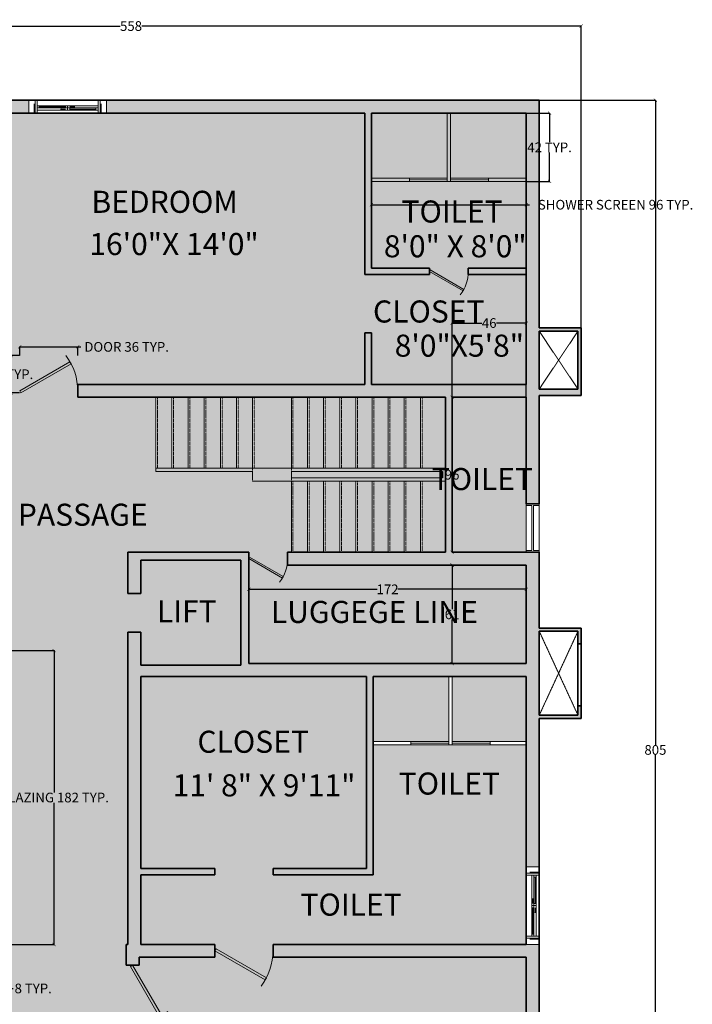
# Model space of a CAD drawing. Units: inches. Extents: x 1704 to 6393, y -157 to 1172.
# Tile 119 of 122: x 4645 to 5062, y 382 to 993. Entities that reach past the tile are written whole.
import ezdxf

# ---------------------------------------------------------------- set-up
doc = ezdxf.new("R2010")
doc.units = ezdxf.units.IN
doc.header["$MEASUREMENT"] = 0
doc.linetypes.add('DASHED', pattern=[0.75, 0.5, -0.25])
doc.linetypes.add('HIDDEN', pattern=[0.375, 0.25, -0.125])
for name, color, linetype, lineweight in [('A-ANNO-DIMS', 7, 'Continuous', 13), ('A-AREA-IDEN', 7, 'Continuous', 18), ('A-FLOR-OPEN-HIDN', 8, 'HIDDEN', 13), ('A-FLOR-STRS-HIDN', 8, 'DASHED', 13), ('A-GLAZ-PATT', 152, 'Continuous', 13), ('A-WALL-PATT', 7, 'Continuous', 13), ('DOORS', 160, 'Continuous', 18), ('GLASS PANEL FASADE', 4, 'Continuous', 18), ('STAIRS', 7, 'Continuous', 18), ('WALLS', 7, 'Continuous', 35), ('WINDOWS', 2, 'Continuous', 18)]:
    doc.layers.add(name, color=color, linetype=linetype, lineweight=lineweight)
doc.layers.add('A-FLOR-PATT', color=7, linetype='Continuous', lineweight=13, true_color=0xf2f2f2)
doc.styles.get("Standard").update_dxf_attribs({"font": 'arial.ttf'})
doc.dimstyles.get("Standard").update_dxf_attribs({"dimtxt": 6, "dimasz": 2, "dimexe": 0.18, "dimexo": 0.0625, "dimgap": 0.09, "dimtad": 0, "dimtih": 1, "dimtoh": 1, "dimdec": 1, "dimzin": 0, "dimdsep": 46, "dimlunit": 3, "dimtxsty": 'Standard', "dimblk": 'ARCHTICK', "dimcen": 0.09, "dimadec": 0, "dimazin": 0, "dimtfac": 1, "dimtdec": 1, "dimtofl": 0, "dimtmove": 0, "dimatfit": 3, "dimfxl": 1, "dimtolj": 1, "dimtzin": 0, "dimarcsym": 0})

# ---------------------------------------------------------------- blocks, each defined once
blk = doc.blocks.new('Door - Left Hung 36 in.')
blk.add_lwpolyline([(0.75, -1.3), (0, 0), (31.18, 18), (31.93, 16.7)], close=True)
blk.add_arc((0, 0), 36, 0, 37.31013)
blk = doc.blocks.new('WIN-SLIDER-48')
for p, q in [((3.83, 8), (0, 8)), ((5.13, 8), (42.87, 8)), ((44.17, 8), (48, 8)), ((3.18, 5.86), (3.18, 0.65)), ((24, 1.95), (5.13, 1.95)), ((6.43, 4.55), (22.7, 4.55)), ((6.43, 3.9), (22.7, 3.9)), ((6.43, 3.25), (22.7, 3.25)), ((22.7, 2.6), (19.9, 2.6)), ((24, 4.55), (42.87, 4.55)), ((25.3, 3.9), (28.1, 3.9)), ((25.3, 3.25), (41.56, 3.25)), ((25.3, 2.6), (41.56, 2.6)), ((25.3, 1.95), (41.56, 1.95)), ((44.82, 5.86), (44.82, 0.65)), ((3.83, 0), (0, 0)), ((5.13, 0), (42.87, 0)), ((44.17, 0), (48, 0))]:
    blk.add_line(p, q)
for points in [[(5.13, 0), (3.83, 0), (3.83, 8), (5.13, 8)], [(42.87, 0), (44.17, 0), (44.17, 8), (42.87, 8)], [(5.13, 3.25), (6.43, 3.25), (6.43, 4.55), (5.13, 4.55)], [(19.57, 2.6), (19.9, 2.8), (19.9, 2.41)], [(22.7, 3.25), (24, 3.25), (24, 4.55), (22.7, 4.55)], [(24, 1.95), (25.3, 1.95), (25.3, 3.25), (24, 3.25)], [(28.43, 3.9), (28.1, 4.1), (28.1, 3.71)], [(41.56, 1.95), (42.87, 1.95), (42.87, 3.25), (41.56, 3.25)]]:
    blk.add_lwpolyline(points, close=True)
blk = doc.blocks.new('WIN-VENT-30')
for p, q in [((0, 0), (0, 30)), ((0, 30), (8, 30)), ((0, 29), (3.5, 29)), ((3.5, 29), (3.5, 1)), ((4.5, 29), (8, 29)), ((4.5, 29), (4.5, 1)), ((8, 30), (8, 0)), ((3.5, 1), (0, 1)), ((8, 1), (4.5, 1)), ((8, 0), (0, 0))]:
    blk.add_line(p, q)
blk = doc.blocks.new('GLAZ-SHOWER-SCREEN-96')
for p, q in [((47, 2), (47, 42.3)), ((49, 2), (49, 42.3)), ((0, 2), (47, 2)), ((23.5, 2), (23.5, 0)), ((23.5, 1), (47, 1)), ((47, 2), (47, 0)), ((49, 2), (96, 2)), ((49, 2), (49, 0)), ((49, 1), (72.5, 1)), ((72.5, 2), (72.5, 0)), ((0, 0), (96, 0))]:
    blk.add_line(p, q)
blk = doc.blocks.new('_ArchTick')
at = {"color": 0, "linetype": 'ByBlock', "const_width": 0.15}
blk.add_lwpolyline([(-0.5, -0.5), (0.5, 0.5)], dxfattribs=at)
blk = doc.blocks.new('*D34')
at = {"layer": 'A-ANNO-DIMS', "color": 0, "lineweight": -2, "transparency": 16777216}
for p, q in [((4645.3, 784.51), (4645.3, 790.02)), ((4645.3, 789.84), (4681.3, 789.84)), ((4681.3, 784.51), (4681.3, 790.02)), ((4681.3, 789.84), (4683.3, 789.84))]:
    blk.add_line(p, q, dxfattribs=at)
at = {"layer": 'Defpoints', "color": 0, "lineweight": -3, "transparency": 16777216}
for p in [(4681.3, 789.84), (4645.3, 784.44), (4681.3, 784.44)]:
    blk.add_point(p, dxfattribs=at)
at = {"layer": 'A-ANNO-DIMS', "color": 0, "lineweight": -2, "transparency": 16777216, "xscale": 2, "yscale": 2, "zscale": 2, "rotation": 180}
blk.add_blockref('_ArchTick', (4645.3, 789.84), dxfattribs=at)
at = {"layer": 'A-ANNO-DIMS', "color": 0, "lineweight": -2, "transparency": 16777216, "xscale": 2, "yscale": 2, "zscale": 2}
blk.add_blockref('_ArchTick', (4681.3, 789.84), dxfattribs=at)
at = {"layer": 'A-ANNO-DIMS', "color": 0, "transparency": 16777216, "insert": (4711.58, 789.84), "char_height": 6, "attachment_point": 5}
blk.add_mtext('\\A1;DOOR 36 TYP.', dxfattribs=at)
blk = doc.blocks.new('*D35')
at = {"layer": 'A-ANNO-DIMS', "color": 0, "lineweight": -2, "transparency": 16777216}
for p, q in [((4645.24, 784.44), (4639.72, 784.44)), ((4639.9, 784.44), (4639.9, 776.04)), ((4639.9, 761.32), (4639.9, 769.73)), ((4645.24, 761.32), (4639.72, 761.32))]:
    blk.add_line(p, q, dxfattribs=at)
at = {"layer": 'Defpoints', "color": 0, "lineweight": -3, "transparency": 16777216}
for p in [(4639.9, 784.44), (4645.3, 784.44), (4645.3, 761.32)]:
    blk.add_point(p, dxfattribs=at)
at = {"layer": 'A-ANNO-DIMS', "color": 0, "lineweight": -2, "transparency": 16777216, "xscale": 2, "yscale": 2, "zscale": 2}
for p, rotation in [((4639.9, 784.44), 90), ((4639.9, 761.32), 270)]:
    blk.add_blockref('_ArchTick', p, dxfattribs=dict(at, rotation=rotation))
at = {"layer": 'A-ANNO-DIMS', "color": 0, "transparency": 16777216, "insert": (4639.9, 772.88), "char_height": 6, "attachment_point": 5}
blk.add_mtext('\\A1;23 TYP.', dxfattribs=at)
blk = doc.blocks.new('*D52')
at = {"layer": 'A-ANNO-DIMS', "color": 0, "lineweight": -2, "transparency": 16777216}
for p, q in [((4639.36, 601.62), (4666.78, 601.62)), ((4666.6, 601.62), (4666.6, 513.82)), ((4666.6, 419.62), (4666.6, 507.43)), ((4639.36, 419.62), (4666.78, 419.62))]:
    blk.add_line(p, q, dxfattribs=at)
at = {"layer": 'Defpoints', "color": 0, "lineweight": -3, "transparency": 16777216}
for p in [(4639.3, 601.62), (4666.6, 601.62), (4639.3, 419.62)]:
    blk.add_point(p, dxfattribs=at)
at = {"layer": 'A-ANNO-DIMS', "color": 0, "lineweight": -2, "transparency": 16777216, "xscale": 2, "yscale": 2, "zscale": 2}
for p, rotation in [((4666.6, 601.62), 90), ((4666.6, 419.62), 270)]:
    blk.add_blockref('_ArchTick', p, dxfattribs=dict(at, rotation=rotation))
at = {"layer": 'A-ANNO-DIMS', "color": 0, "transparency": 16777216, "insert": (4666.6, 510.62), "char_height": 6, "attachment_point": 5}
blk.add_mtext('\\A1;GLAZING 182 TYP.', dxfattribs=at)
blk = doc.blocks.new('*D53')
at = {"layer": 'A-ANNO-DIMS', "color": 0, "lineweight": -2, "transparency": 16777216}
for p, q in [((4631.3, 419.56), (4631.3, 392.14)), ((4639.3, 419.56), (4639.3, 392.14)), ((4631.3, 392.32), (4639.3, 392.32)), ((4639.3, 392.32), (4641.3, 392.32))]:
    blk.add_line(p, q, dxfattribs=at)
at = {"layer": 'Defpoints', "color": 0, "lineweight": -3, "transparency": 16777216}
for p in [(4631.3, 419.62), (4639.3, 419.62), (4639.3, 392.32)]:
    blk.add_point(p, dxfattribs=at)
at = {"layer": 'A-ANNO-DIMS', "color": 0, "lineweight": -2, "transparency": 16777216, "xscale": 2, "yscale": 2, "zscale": 2, "rotation": 180}
blk.add_blockref('_ArchTick', (4631.3, 392.32), dxfattribs=at)
at = {"layer": 'A-ANNO-DIMS', "color": 0, "lineweight": -2, "transparency": 16777216, "xscale": 2, "yscale": 2, "zscale": 2}
blk.add_blockref('_ArchTick', (4639.3, 392.32), dxfattribs=at)
at = {"layer": 'A-ANNO-DIMS', "color": 0, "transparency": 16777216, "insert": (4653.67, 392.32), "char_height": 6, "attachment_point": 5}
blk.add_mtext('\\A1;8 TYP.', dxfattribs=at)
blk = doc.blocks.new('*D54')
at = {"layer": 'A-ANNO-DIMS', "color": 0, "lineweight": -2, "transparency": 16777216}
for p, q in [((4863.3, 892.26), (4863.3, 877.74)), ((4959.3, 892.26), (4959.3, 877.74)), ((4863.3, 877.92), (4959.3, 877.92)), ((4959.3, 877.92), (4961.3, 877.92))]:
    blk.add_line(p, q, dxfattribs=at)
at = {"layer": 'Defpoints', "color": 0, "lineweight": -3, "transparency": 16777216}
for p in [(4863.3, 892.32), (4959.3, 892.32), (4959.3, 877.92)]:
    blk.add_point(p, dxfattribs=at)
at = {"layer": 'A-ANNO-DIMS', "color": 0, "lineweight": -2, "transparency": 16777216, "xscale": 2, "yscale": 2, "zscale": 2, "rotation": 180}
blk.add_blockref('_ArchTick', (4863.3, 877.92), dxfattribs=at)
at = {"layer": 'A-ANNO-DIMS', "color": 0, "lineweight": -2, "transparency": 16777216, "xscale": 2, "yscale": 2, "zscale": 2}
blk.add_blockref('_ArchTick', (4959.3, 877.92), dxfattribs=at)
at = {"layer": 'A-ANNO-DIMS', "color": 0, "transparency": 16777216, "insert": (5014.63, 877.92), "char_height": 6, "attachment_point": 5}
blk.add_mtext('\\A1;SHOWER SCREEN 96 TYP.', dxfattribs=at)
blk = doc.blocks.new('*D55')
at = {"layer": 'A-ANNO-DIMS', "color": 0, "lineweight": -2, "transparency": 16777216}
for p, q in [((4959.36, 934.62), (4973.88, 934.62)), ((4973.7, 934.62), (4973.7, 916.58)), ((4973.7, 892.32), (4973.7, 910.37)), ((4959.36, 892.32), (4973.88, 892.32))]:
    blk.add_line(p, q, dxfattribs=at)
at = {"layer": 'Defpoints', "color": 0, "lineweight": -3, "transparency": 16777216}
for p in [(4959.3, 934.62), (4973.7, 934.62), (4959.3, 892.32)]:
    blk.add_point(p, dxfattribs=at)
at = {"layer": 'A-ANNO-DIMS', "color": 0, "lineweight": -2, "transparency": 16777216, "xscale": 2, "yscale": 2, "zscale": 2}
for p, rotation in [((4973.7, 934.62), 90), ((4973.7, 892.32), 270)]:
    blk.add_blockref('_ArchTick', p, dxfattribs=dict(at, rotation=rotation))
at = {"layer": 'A-ANNO-DIMS', "color": 0, "transparency": 16777216, "insert": (4973.7, 913.47), "char_height": 6, "attachment_point": 5}
blk.add_mtext('\\A1;42 TYP.', dxfattribs=at)
blk = doc.blocks.new('*D107')
at = {"layer": 'A-ANNO-DIMS', "color": 0, "lineweight": -2, "transparency": 16777216}
for p, q in [((4435.3, 942.69), (4435.3, 988.8)), ((4435.3, 988.62), (4707.58, 988.62)), ((4993.3, 988.62), (4721.02, 988.62)), ((4993.3, 801.69), (4993.3, 988.8))]:
    blk.add_line(p, q, dxfattribs=at)
at = {"layer": 'Defpoints', "color": 0, "lineweight": -3, "transparency": 16777216}
for p in [(4993.3, 988.62), (4435.3, 942.62), (4993.3, 801.62)]:
    blk.add_point(p, dxfattribs=at)
at = {"layer": 'A-ANNO-DIMS', "color": 0, "lineweight": -2, "transparency": 16777216, "xscale": 2, "yscale": 2, "zscale": 2, "rotation": 180}
blk.add_blockref('_ArchTick', (4435.3, 988.62), dxfattribs=at)
at = {"layer": 'A-ANNO-DIMS', "color": 0, "lineweight": -2, "transparency": 16777216, "xscale": 2, "yscale": 2, "zscale": 2}
blk.add_blockref('_ArchTick', (4993.3, 988.62), dxfattribs=at)
at = {"layer": 'A-ANNO-DIMS', "color": 0, "transparency": 16777216, "insert": (4714.3, 988.62), "char_height": 6, "attachment_point": 5}
blk.add_mtext('\\A1;558', dxfattribs=at)
blk = doc.blocks.new('*D108')
at = {"layer": 'A-ANNO-DIMS', "color": 0, "lineweight": -2, "transparency": 16777216}
for p, q in [((4967.36, 942.62), (5039.48, 942.62)), ((5039.3, 942.62), (5039.3, 543.28)), ((5039.3, 137.62), (5039.3, 536.97)), ((4967.36, 137.62), (5039.48, 137.62))]:
    blk.add_line(p, q, dxfattribs=at)
at = {"layer": 'Defpoints', "color": 0, "lineweight": -3, "transparency": 16777216}
for p in [(4967.3, 942.62), (5039.3, 942.62), (4967.3, 137.62)]:
    blk.add_point(p, dxfattribs=at)
at = {"layer": 'A-ANNO-DIMS', "color": 0, "lineweight": -2, "transparency": 16777216, "xscale": 2, "yscale": 2, "zscale": 2}
for p, rotation in [((5039.3, 942.62), 90), ((5039.3, 137.62), 270)]:
    blk.add_blockref('_ArchTick', p, dxfattribs=dict(at, rotation=rotation))
at = {"layer": 'A-ANNO-DIMS', "color": 0, "transparency": 16777216, "insert": (5039.3, 540.12), "char_height": 6, "attachment_point": 5}
blk.add_mtext('\\A1;805', dxfattribs=at)
blk = doc.blocks.new('*D115')
at = {"layer": 'A-ANNO-DIMS', "color": 0, "lineweight": -2, "transparency": 16777216}
for p, q in [((4787.3, 593.69), (4787.3, 639.8)), ((4787.3, 639.62), (4866.9, 639.62)), ((4959.3, 639.62), (4879.71, 639.62)), ((4959.3, 593.69), (4959.3, 639.8))]:
    blk.add_line(p, q, dxfattribs=at)
at = {"layer": 'Defpoints', "color": 0, "lineweight": -3, "transparency": 16777216}
for p in [(4959.3, 639.62), (4787.3, 593.62), (4959.3, 593.62)]:
    blk.add_point(p, dxfattribs=at)
at = {"layer": 'A-ANNO-DIMS', "color": 0, "lineweight": -2, "transparency": 16777216, "xscale": 2, "yscale": 2, "zscale": 2, "rotation": 180}
blk.add_blockref('_ArchTick', (4787.3, 639.62), dxfattribs=at)
at = {"layer": 'A-ANNO-DIMS', "color": 0, "lineweight": -2, "transparency": 16777216, "xscale": 2, "yscale": 2, "zscale": 2}
blk.add_blockref('_ArchTick', (4959.3, 639.62), dxfattribs=at)
at = {"layer": 'A-ANNO-DIMS', "color": 0, "transparency": 16777216, "insert": (4873.3, 639.62), "char_height": 6, "attachment_point": 5}
blk.add_mtext('\\A1;172', dxfattribs=at)
blk = doc.blocks.new('*D116')
at = {"layer": 'A-ANNO-DIMS', "color": 0, "lineweight": -2, "transparency": 16777216}
for p, q in [((4959.24, 654.62), (4913.12, 654.62)), ((4913.3, 654.62), (4913.3, 627.28)), ((4913.3, 593.62), (4913.3, 620.97)), ((4959.24, 593.62), (4913.12, 593.62))]:
    blk.add_line(p, q, dxfattribs=at)
at = {"layer": 'Defpoints', "color": 0, "lineweight": -3, "transparency": 16777216}
for p in [(4913.3, 654.62), (4959.3, 654.62), (4959.3, 593.62)]:
    blk.add_point(p, dxfattribs=at)
at = {"layer": 'A-ANNO-DIMS', "color": 0, "lineweight": -2, "transparency": 16777216, "xscale": 2, "yscale": 2, "zscale": 2}
for p, rotation in [((4913.3, 654.62), 90), ((4913.3, 593.62), 270)]:
    blk.add_blockref('_ArchTick', p, dxfattribs=dict(at, rotation=rotation))
at = {"layer": 'A-ANNO-DIMS', "color": 0, "transparency": 16777216, "insert": (4913.3, 624.12), "char_height": 6, "attachment_point": 5}
blk.add_mtext('\\A1;61', dxfattribs=at)
blk = doc.blocks.new('*D117')
at = {"layer": 'A-ANNO-DIMS', "color": 0, "lineweight": -2, "transparency": 16777216}
for p, q in [((4959.24, 758.62), (4913.12, 758.62)), ((4913.3, 758.62), (4913.3, 713.78)), ((4913.3, 662.62), (4913.3, 707.47)), ((4959.24, 662.62), (4913.12, 662.62))]:
    blk.add_line(p, q, dxfattribs=at)
at = {"layer": 'Defpoints', "color": 0, "lineweight": -3, "transparency": 16777216}
for p in [(4913.3, 758.62), (4959.3, 758.62), (4959.3, 662.62)]:
    blk.add_point(p, dxfattribs=at)
at = {"layer": 'A-ANNO-DIMS', "color": 0, "lineweight": -2, "transparency": 16777216, "xscale": 2, "yscale": 2, "zscale": 2}
for p, rotation in [((4913.3, 758.62), 90), ((4913.3, 662.62), 270)]:
    blk.add_blockref('_ArchTick', p, dxfattribs=dict(at, rotation=rotation))
at = {"layer": 'A-ANNO-DIMS', "color": 0, "transparency": 16777216, "insert": (4913.3, 710.62), "char_height": 6, "attachment_point": 5}
blk.add_mtext('\\A1;96', dxfattribs=at)
blk = doc.blocks.new('*D118')
at = {"layer": 'A-ANNO-DIMS', "color": 0, "lineweight": -2, "transparency": 16777216}
for p, q in [((4913.3, 758.69), (4913.3, 804.8)), ((4913.3, 804.62), (4931.79, 804.62)), ((4959.3, 804.62), (4940.81, 804.62)), ((4959.3, 758.69), (4959.3, 804.8))]:
    blk.add_line(p, q, dxfattribs=at)
at = {"layer": 'Defpoints', "color": 0, "lineweight": -3, "transparency": 16777216}
for p in [(4959.3, 804.62), (4913.3, 758.62), (4959.3, 758.62)]:
    blk.add_point(p, dxfattribs=at)
at = {"layer": 'A-ANNO-DIMS', "color": 0, "lineweight": -2, "transparency": 16777216, "xscale": 2, "yscale": 2, "zscale": 2, "rotation": 180}
blk.add_blockref('_ArchTick', (4913.3, 804.62), dxfattribs=at)
at = {"layer": 'A-ANNO-DIMS', "color": 0, "lineweight": -2, "transparency": 16777216, "xscale": 2, "yscale": 2, "zscale": 2}
blk.add_blockref('_ArchTick', (4959.3, 804.62), dxfattribs=at)
at = {"layer": 'A-ANNO-DIMS', "color": 0, "transparency": 16777216, "insert": (4936.3, 804.62), "char_height": 6, "attachment_point": 5}
blk.add_mtext('\\A1;46', dxfattribs=at)
blk = doc.blocks.new('*D138')
at = {"layer": 'A-ANNO-DIMS', "color": 0, "lineweight": -2, "transparency": 16777216}
for p, q in [((4715.21, 406.69), (4715.39, 406.69)), ((4715.3, 406.6), (4715.3, 406.78)), ((4733.73, 352.12), (4726.82, 372.59)), ((4735.73, 352.12), (4733.73, 352.12))]:
    blk.add_line(p, q, dxfattribs=at)
at = {"layer": 'Defpoints', "color": 0, "lineweight": -3, "transparency": 16777216}
for p in [(4715.3, 406.69), (4726.82, 372.59)]:
    blk.add_point(p, dxfattribs=at)
at = {"layer": 'A-ANNO-DIMS', "color": 0, "lineweight": -2, "transparency": 16777216, "xscale": 2, "yscale": 2, "zscale": 2, "rotation": 108.6557587224779}
blk.add_blockref('_ArchTick', (4726.82, 372.59), dxfattribs=at)
at = {"layer": 'A-ANNO-DIMS', "color": 0, "transparency": 16777216, "insert": (4749.48, 352.12), "char_height": 6, "attachment_point": 5}
blk.add_mtext('\\A1;2X R36', dxfattribs=at)

msp = doc.modelspace()

# ---------------------------------------------------------------- hatches: boundary and pattern name
at = {"layer": 'A-FLOR-PATT', "transparency": 33554516}
h = msp.add_hatch(color=256, dxfattribs=at)
h.dxf.hatch_style = 1
h.paths.add_polyline_path([(4859.3, 934.624), (4639.3, 934.624), (4639.3, 766.624), (4645.3, 766.624), (4645.3, 762.624), (4676.477, 780.624), (4677.227, 779.325), (4677.2, 779.309, -0.0929107), (4681.077, 766.624), (4687.3, 766.624), (4859.3, 766.624), (4859.3, 798.624), (4863.3, 798.624), (4863.3, 766.624), (4875.3, 766.624), (4959.3, 766.624), (4959.3, 834.624), (4923.217, 834.624, -0.0999534), (4920.567, 825.5), (4920.585, 825.49), (4920.085, 824.624), (4899.3, 836.624), (4899.3, 834.624), (4863.3, 834.624), (4859.3, 834.624)])
h.paths.add_polyline_path([(4631.3, 890.624), (4443.3, 890.624), (4443.3, 722.624), (4559.3, 722.624), (4559.3, 718.624), (4535.3, 718.624), (4535.3, 712.624), (4531.3, 712.624), (4532.383, 711.999), (4517.396, 686.04, 0.1210664), (4531.3, 682.624), (4535.3, 682.624), (4535.3, 609.624), (4631.3, 609.624), (4631.3, 718.624), (4595.3, 718.624), (4595.3, 722.624), (4631.3, 722.624), (4637.3, 722.624, -0.1140277), (4621.609, 726.711), (4621.593, 726.684), (4620.293, 727.435), (4638.3, 758.624), (4631.3, 758.624)])
h.paths.add_polyline_path([(4531.3, 712.624), (4527.3, 712.624), (4527.3, 718.624), (4443.3, 718.624), (4443.3, 609.624), (4527.3, 609.624), (4527.3, 682.891, -0.0872676), (4517.396, 686.04), (4517.383, 686.018), (4516.3, 686.643)], flags=17)
h.paths.add_polyline_path([(4631.3, 601.624), (4537.3, 510.624), (4631.3, 419.624)], flags=17)
h.paths.add_polyline_path([(4537.3, 510.624), (4443.3, 419.624), (4453.75, 419.624), (4617.46, 419.624), (4631.3, 419.624)], flags=17)
h.paths.add_polyline_path([(4443.3, 601.624), (4443.3, 419.624), (4537.3, 510.624)], flags=17)
h.paths.add_polyline_path([(4631.3, 601.624), (4443.3, 601.624), (4537.3, 510.624)], flags=17)
h.paths.add_polyline_path([(4637.3, 370.694), (4711.3, 370.694), (4715.3, 370.694, 0.1210664), (4731.986, 374.795), (4713.568, 406.694), (4711.3, 406.694), (4711.3, 419.624), (4712.3, 419.624), (4712.3, 613.124), (4720.3, 613.124), (4720.3, 592.624), (4782.3, 592.624), (4782.3, 657.624), (4720.3, 657.624), (4720.3, 637.124), (4712.3, 637.124), (4712.3, 662.624), (4787.3, 662.624), (4787.3, 654.624), (4787.3, 593.624), (4959.3, 593.624), (4959.3, 654.624), (4811.3, 654.624), (4811.3, 662.624), (4813.69, 662.624), (4813.69, 706.624), (4789.69, 706.624), (4789.69, 712.624), (4729.69, 712.624), (4729.69, 714.624), (4729.69, 758.624), (4681.3, 758.624), (4681.3, 762.624, 0.1210664), (4677.2, 779.309), (4645.3, 760.892), (4645.3, 758.624), (4638.3, 758.624), (4639.6, 757.873), (4621.609, 726.711, 0.1140277), (4637.3, 722.624), (4639.3, 722.624), (4639.3, 601.624), (4639.3, 419.624), (4639.3, 411.624), (4617.46, 411.624), (4453.75, 411.624), (4443.3, 411.624), (4443.3, 249.624), (4637.3, 249.624)])
h.paths.add_polyline_path([(4813.69, 758.624), (4790.69, 758.624), (4790.69, 714.624), (4813.69, 714.624)], flags=17)
h.paths.add_polyline_path([(4789.69, 758.624), (4780.69, 758.624), (4780.69, 714.624), (4789.69, 714.624)], flags=17)
h.paths.add_polyline_path([(4779.69, 758.624), (4770.69, 758.624), (4770.69, 714.624), (4779.69, 714.624)], flags=17)
h.paths.add_polyline_path([(4769.69, 758.624), (4760.69, 758.624), (4760.69, 714.624), (4769.69, 714.624)], flags=17)
h.paths.add_polyline_path([(4759.69, 758.624), (4750.69, 758.624), (4750.69, 714.624), (4759.69, 714.624)], flags=17)
h.paths.add_polyline_path([(4749.69, 758.624), (4740.69, 758.624), (4740.69, 714.624), (4749.69, 714.624)], flags=17)
h.paths.add_polyline_path([(4739.69, 758.624), (4730.69, 758.624), (4730.69, 714.624), (4739.69, 714.624)], flags=17)
h.paths.add_polyline_path([(4823.69, 758.624), (4814.69, 758.624), (4814.69, 714.624), (4823.69, 714.624)], flags=17)
h.paths.add_polyline_path([(4833.69, 758.624), (4824.69, 758.624), (4824.69, 714.624), (4833.69, 714.624)], flags=17)
h.paths.add_polyline_path([(4843.69, 758.624), (4834.69, 758.624), (4834.69, 714.624), (4843.69, 714.624)], flags=17)
h.paths.add_polyline_path([(4909.3, 706.624), (4894.69, 706.624), (4894.69, 662.624), (4909.3, 662.624)], flags=17)
h.paths.add_polyline_path([(4883.69, 706.624), (4874.69, 706.624), (4874.69, 662.624), (4883.69, 662.624)], flags=17)
h.paths.add_polyline_path([(4853.69, 706.624), (4844.69, 706.624), (4844.69, 662.624), (4853.69, 662.624)], flags=17)
h.paths.add_polyline_path([(4833.69, 706.624), (4824.69, 706.624), (4824.69, 662.624), (4833.69, 662.624)], flags=17)
h.paths.add_polyline_path([(4823.69, 706.624), (4814.69, 706.624), (4814.69, 662.624), (4823.69, 662.624)], flags=17)
h.paths.add_polyline_path([(4843.69, 706.624), (4834.69, 706.624), (4834.69, 662.624), (4843.69, 662.624)], flags=17)
h.paths.add_polyline_path([(4863.69, 706.624), (4854.69, 706.624), (4854.69, 662.624), (4863.69, 662.624)], flags=17)
h.paths.add_polyline_path([(4873.69, 706.624), (4864.69, 706.624), (4864.69, 662.624), (4873.69, 662.624)], flags=17)
h.paths.add_polyline_path([(4893.69, 706.624), (4884.69, 706.624), (4884.69, 662.624), (4893.69, 662.624)], flags=17)
h.paths.add_polyline_path([(4853.69, 758.624), (4844.69, 758.624), (4844.69, 714.624), (4853.69, 714.624)], flags=17)
h.paths.add_polyline_path([(4873.69, 758.624), (4864.69, 758.624), (4864.69, 714.624), (4873.69, 714.624)], flags=17)
h.paths.add_polyline_path([(4893.69, 758.624), (4884.69, 758.624), (4884.69, 714.624), (4893.69, 714.624)], flags=17)
h.paths.add_polyline_path([(4909.3, 758.624), (4894.69, 758.624), (4894.69, 714.624), (4909.3, 714.624)], flags=17)
h.paths.add_polyline_path([(4863.69, 758.624), (4854.69, 758.624), (4854.69, 714.624), (4863.69, 714.624)], flags=17)
h.paths.add_polyline_path([(4883.69, 758.624), (4874.69, 758.624), (4874.69, 714.624), (4883.69, 714.624)], flags=17)
h.paths.add_polyline_path([(4907.3, 712.624), (4813.69, 712.624), (4813.69, 708.624), (4907.3, 708.624)], flags=17)
at = {"layer": 'A-FLOR-PATT', "transparency": 33554511}
h = msp.add_hatch(color=256, dxfattribs=at)
h.dxf.hatch_style = 1
h.paths.add_polyline_path([(4860.3, 585.624), (4839.3, 585.624), (4720.3, 585.624), (4720.3, 466.624), (4766.3, 466.624), (4766.3, 462.624), (4720.3, 462.624), (4720.3, 419.624), (4766.3, 419.624), (4766.3, 415.624), (4767.05, 416.923), (4798.2, 398.938, 0.1210664), (4802.3, 415.624), (4802.3, 419.624), (4959.3, 419.624), (4959.3, 423.456), (4959.3, 424.757), (4959.3, 462.49), (4959.3, 463.791), (4959.3, 467.624), (4959.3, 543.32), (4864.3, 543.32), (4864.3, 462.624), (4802.3, 462.624), (4802.3, 466.624), (4860.3, 466.624)], flags=17)
h.paths.add_polyline_path([(4959.3, 411.624), (4802.077, 411.624, -0.0929107), (4798.2, 398.938), (4767.05, 416.923), (4766.3, 415.624), (4766.3, 411.624), (4719.3, 411.624), (4719.3, 406.694), (4711.3, 406.694), (4711.3, 419.624), (4712.3, 419.624), (4712.3, 613.124), (4720.3, 613.124), (4720.3, 592.624), (4782.3, 592.624), (4782.3, 657.624), (4720.3, 657.624), (4720.3, 637.124), (4712.3, 637.124), (4712.3, 662.624), (4787.3, 662.624), (4787.3, 654.624), (4787.3, 593.624), (4959.3, 593.624), (4959.3, 654.624), (4811.3, 654.624), (4811.3, 662.624), (4813.69, 662.624), (4813.69, 706.624), (4789.69, 706.624), (4789.69, 712.624), (4729.69, 712.624), (4729.69, 714.624), (4729.69, 758.624), (4681.3, 758.624), (4681.3, 766.624), (4687.3, 766.624), (4859.3, 766.624), (4859.3, 798.624), (4863.3, 798.624), (4863.3, 766.624), (4875.3, 766.624), (4959.3, 766.624), (4959.3, 834.624), (4923.3, 834.624), (4923.3, 838.624), (4959.3, 838.624), (4959.3, 892.32), (4863.3, 892.32), (4863.3, 838.624), (4899.3, 838.624), (4899.3, 834.624), (4863.3, 834.624), (4859.3, 834.624), (4859.3, 934.624), (4639.3, 934.624), (4639.3, 766.624), (4645.3, 766.624), (4645.3, 758.624), (4631.3, 758.624), (4631.3, 890.624), (4443.3, 890.624), (4443.3, 722.624), (4559.3, 722.624), (4559.3, 718.624), (4535.3, 718.624), (4535.3, 712.624), (4527.3, 712.624), (4527.3, 718.624), (4443.3, 718.624), (4443.3, 609.624), (4527.3, 609.624), (4527.3, 682.624), (4535.3, 682.624), (4535.3, 609.624), (4631.3, 609.624), (4631.3, 718.624), (4595.3, 718.624), (4595.3, 722.624), (4631.3, 722.624), (4639.3, 722.624), (4639.3, 601.624), (4639.3, 419.624), (4639.3, 411.624), (4617.46, 411.624), (4453.75, 411.624), (4443.3, 411.624), (4443.3, 249.624), (4637.3, 249.624), (4637.3, 370.694), (4711.3, 370.694), (4719.3, 370.694), (4719.3, 145.624), (4959.3, 145.624), (4959.3, 265.624)])
h.paths.add_polyline_path([(4645.3, 362.694), (4645.3, 249.624), (4678.295, 306.15)], flags=17)
h.paths.add_polyline_path([(4711.3, 362.694), (4645.3, 362.694), (4678.295, 306.15)], flags=17)
h.paths.add_polyline_path([(4711.3, 362.694), (4678.295, 306.15), (4711.279, 249.624), (4711.3, 249.624)], flags=17)
at = {"layer": 'A-FLOR-PATT', "transparency": 33554559}
h = msp.add_hatch(color=256, dxfattribs=at)
h.dxf.hatch_style = 1
h.paths.add_polyline_path([(4959.3, 892.32), (4863.3, 892.32), (4863.3, 838.624), (4899.3, 838.624), (4899.3, 836.624), (4899.8, 837.49), (4920.567, 825.5, 0.1210664), (4923.3, 836.624), (4923.3, 838.624), (4959.3, 838.624)])
h.paths.add_polyline_path([(4910.3, 934.624), (4863.3, 934.624), (4863.3, 894.32), (4910.3, 894.32)])
h.paths.add_polyline_path([(4959.3, 934.624), (4912.3, 934.624), (4912.3, 894.32), (4959.3, 894.32)])
h = msp.add_hatch(color=256, dxfattribs=at)
h.dxf.hatch_style = 1
h.paths.add_polyline_path([(4959.3, 758.624), (4913.3, 758.624), (4913.3, 662.624), (4959.3, 662.624), (4959.3, 692.624)])
h = msp.add_hatch(color=256, dxfattribs=at)
h.dxf.hatch_style = 1
h.paths.add_polyline_path([(4911.3, 585.624), (4864.3, 585.624), (4864.3, 545.32), (4911.3, 545.32)])
h.paths.add_polyline_path([(4959.3, 585.624), (4913.3, 585.624), (4913.3, 545.32), (4959.3, 545.32)])
at = {"layer": 'A-GLAZ-PATT', "transparency": 33554559}
h = msp.add_hatch(color=256, dxfattribs=at)
h.dxf.hatch_style = 1
h.paths.add_polyline_path([(4886.8, 894.32), (4863.3, 894.32), (4863.3, 892.32), (4886.8, 892.32)])
h.paths.add_polyline_path([(4912.3, 934.624), (4910.3, 934.624), (4910.3, 894.32), (4910.3, 892.32), (4912.3, 892.32), (4912.3, 894.32)])
h = msp.add_hatch(color=256, dxfattribs=at)
h.dxf.hatch_style = 1
h.paths.add_polyline_path([(4959.3, 894.32), (4935.8, 894.32), (4935.8, 892.32), (4959.3, 892.32)])
at = {"layer": 'A-WALL-PATT'}
h = msp.add_hatch(color=256, dxfattribs=at)
h.dxf.hatch_style = 1
h.paths.add_polyline_path([(4967.3, 942.624), (4699.009, 942.624), (4699.009, 934.624), (4859.3, 934.624), (4859.3, 834.624), (4863.3, 834.624), (4899.3, 834.624), (4899.3, 838.624), (4863.3, 838.624), (4863.3, 934.624), (4959.3, 934.624), (4959.3, 901.624), (4959.3, 834.624), (4959.3, 766.624), (4863.3, 766.624), (4863.3, 798.624), (4859.3, 798.624), (4859.3, 766.624), (4687.3, 766.624), (4681.3, 766.624), (4681.3, 758.624), (4909.3, 758.624), (4909.3, 662.624), (4811.3, 662.624), (4811.3, 654.624), (4959.3, 654.624), (4959.3, 593.624), (4787.3, 593.624), (4787.3, 654.624), (4787.3, 662.624), (4712.3, 662.624), (4712.3, 637.124), (4720.3, 637.124), (4720.3, 657.624), (4782.3, 657.624), (4782.3, 592.624), (4720.3, 592.624), (4720.3, 613.124), (4712.3, 613.124), (4712.3, 419.624), (4711.3, 419.624), (4711.3, 406.694), (4719.3, 406.694), (4719.3, 411.624), (4766.3, 411.624), (4766.3, 419.624), (4720.3, 419.624), (4720.3, 462.624), (4766.3, 462.624), (4766.3, 466.624), (4720.3, 466.624), (4720.3, 585.624), (4839.3, 585.624), (4860.3, 585.624), (4860.3, 466.624), (4802.3, 466.624), (4802.3, 462.624), (4864.3, 462.624), (4864.3, 585.624), (4959.3, 585.624), (4959.3, 542.624), (4959.3, 467.624), (4967.3, 467.624), (4967.3, 559.624), (4993.3, 559.624), (4993.3, 567.435), (4991.3, 567.435), (4991.3, 561.624), (4967.3, 561.624), (4967.3, 613.624), (4991.3, 613.624), (4991.3, 605.789), (4993.3, 605.789), (4993.3, 615.624), (4967.3, 615.624), (4967.3, 654.624), (4967.3, 662.624), (4959.3, 662.624), (4913.3, 662.624), (4913.3, 758.624), (4959.3, 758.624), (4959.3, 692.624), (4967.3, 692.624), (4967.3, 759.624), (4993.3, 759.624), (4993.3, 801.624), (4967.3, 801.624)])
h.paths.add_polyline_path([(4967.3, 799.624), (4991.3, 799.624), (4991.3, 763.624), (4967.3, 763.624)], flags=16)
h.paths.add_polyline_path([(4443.3, 718.624), (4527.3, 718.624), (4527.3, 712.624), (4535.3, 712.624), (4535.3, 718.624), (4559.3, 718.624), (4559.3, 722.624), (4443.3, 722.624), (4435.3, 722.624), (4435.3, 601.624), (4443.3, 601.624), (4639.3, 601.624), (4639.3, 722.624), (4631.3, 722.624), (4595.3, 722.624), (4595.3, 718.624), (4631.3, 718.624), (4631.3, 609.624), (4535.3, 609.624), (4535.3, 682.624), (4527.3, 682.624), (4527.3, 609.624), (4443.3, 609.624)])
h.paths.add_polyline_path([(4443.3, 890.624), (4489.3, 890.624), (4489.3, 898.624), (4443.3, 898.624), (4443.3, 934.624), (4455.446, 934.624), (4455.446, 942.624), (4435.3, 942.624), (4435.3, 794.624), (4443.3, 794.624)])
h.paths.add_polyline_path([(4639.3, 934.624), (4651.009, 934.624), (4651.009, 942.624), (4635.3, 942.624), (4619.155, 942.624), (4619.155, 934.624), (4631.3, 934.624), (4631.3, 898.624), (4585.3, 898.624), (4585.3, 890.624), (4631.3, 890.624), (4631.3, 758.624), (4645.3, 758.624), (4645.3, 766.624), (4639.3, 766.624)])
h.paths.add_polyline_path([(4967.3, 265.624), (4967.3, 309.624), (4959.3, 309.624), (4959.3, 265.624), (4959.3, 145.624), (4719.3, 145.624), (4719.3, 370.694), (4711.3, 370.694), (4711.3, 249.624), (4699.3, 249.624), (4651.3, 249.624), (4639.3, 249.624), (4585.307, 249.624), (4585.307, 241.624), (4639.3, 241.624), (4651.3, 241.624), (4699.3, 241.624), (4711.3, 241.624), (4711.3, 137.624), (4719.3, 137.624), (4959.3, 137.624), (4967.3, 137.624)])
h.paths.add_polyline_path([(4489.307, 249.624), (4435.313, 249.624), (4435.313, 241.624), (4489.307, 241.624)])
h.paths.add_polyline_path([(4967.3, 419.624), (4959.3, 419.624), (4802.3, 419.624), (4802.3, 411.624), (4959.3, 411.624), (4959.3, 381.624), (4967.3, 381.624)])
h.paths.add_polyline_path([(4967.3, 381.624), (4959.3, 381.624), (4959.3, 376.851), (4967.3, 376.851)])
h.paths.add_polyline_path([(4967.3, 314.396), (4959.3, 314.396), (4959.3, 309.624), (4967.3, 309.624)], flags=17)
h.paths.add_polyline_path([(4959.3, 838.624), (4923.3, 838.624), (4923.3, 834.624), (4959.3, 834.624)], flags=17)
h = msp.add_hatch(color=256, dxfattribs=at)
h.dxf.hatch_style = 1
h.paths.add_polyline_path([(4813.69, 714.624), (4789.69, 714.624), (4789.69, 706.624), (4813.69, 706.624)])
h.paths.add_polyline_path([(4909.3, 714.624), (4813.69, 714.624), (4813.69, 712.624), (4907.3, 712.624), (4907.3, 708.624), (4813.69, 708.624), (4813.69, 706.624), (4909.3, 706.624)])
h.paths.add_polyline_path([(4789.69, 714.624), (4729.69, 714.624), (4729.69, 712.624), (4789.69, 712.624)])

# ---------------------------------------------------------------- linework, layer by layer
at = {"layer": 'A-FLOR-OPEN-HIDN'}
for p, q in [((4967.3, 763.624), (4991.3, 799.624)), ((4967.3, 799.624), (4991.3, 763.624)), ((4967.3, 561.624), (4991.3, 613.624)), ((4967.3, 613.624), (4991.3, 561.624))]:
    msp.add_line(p, q, dxfattribs=at)
at = {"layer": 'A-FLOR-STRS-HIDN'}
for p, q in [((4730.69, 714.624), (4730.69, 758.624)), ((4740.69, 714.624), (4740.69, 758.624)), ((4750.69, 714.624), (4750.69, 758.624)), ((4760.69, 714.624), (4760.69, 758.624)), ((4770.69, 714.624), (4770.69, 758.624)), ((4780.69, 714.624), (4780.69, 758.624)), ((4790.69, 714.624), (4790.69, 758.624)), ((4814.69, 714.624), (4814.69, 758.624)), ((4824.69, 714.624), (4824.69, 758.624)), ((4834.69, 714.624), (4834.69, 758.624)), ((4844.69, 714.624), (4844.69, 758.624)), ((4854.69, 714.624), (4854.69, 758.624)), ((4864.69, 714.624), (4864.69, 758.624)), ((4874.69, 714.624), (4874.69, 758.624)), ((4884.69, 714.624), (4884.69, 758.624)), ((4894.69, 714.624), (4894.69, 758.624)), ((4789.69, 714.624), (4789.69, 706.624)), ((4813.69, 706.624), (4813.69, 714.624)), ((4814.69, 706.624), (4814.69, 662.624)), ((4824.69, 706.624), (4824.69, 662.624)), ((4834.69, 706.624), (4834.69, 662.624)), ((4844.69, 706.624), (4844.69, 662.624)), ((4854.69, 706.624), (4854.69, 662.624)), ((4864.69, 706.624), (4864.69, 662.624)), ((4874.69, 706.624), (4874.69, 662.624)), ((4884.69, 706.624), (4884.69, 662.624)), ((4894.69, 706.624), (4894.69, 662.624))]:
    msp.add_line(p, q, dxfattribs=at)
at = {"layer": 'GLASS PANEL FASADE'}
for p, q in [((4911.3, 545.32), (4911.3, 585.624)), ((4913.3, 545.32), (4913.3, 585.624)), ((4864.3, 545.32), (4911.3, 545.32)), ((4864.3, 543.32), (4959.3, 543.32)), ((4887.8, 543.32), (4887.8, 545.32)), ((4887.8, 544.32), (4911.3, 544.32)), ((4911.3, 545.32), (4911.3, 543.32)), ((4913.3, 545.32), (4959.3, 545.32)), ((4913.3, 545.32), (4913.3, 543.32)), ((4913.3, 544.32), (4936.8, 544.32)), ((4936.8, 543.32), (4936.8, 545.32))]:
    msp.add_line(p, q, dxfattribs=at)
at = {"layer": 'STAIRS'}
for p, q in [((4729.69, 714.624), (4729.69, 758.624)), ((4739.69, 714.624), (4739.69, 758.624)), ((4749.69, 714.624), (4749.69, 758.624)), ((4759.69, 714.624), (4759.69, 758.624)), ((4769.69, 714.624), (4769.69, 758.624)), ((4779.69, 714.624), (4779.69, 758.624)), ((4789.69, 714.624), (4789.69, 758.624)), ((4813.69, 714.624), (4813.69, 758.624)), ((4823.69, 714.624), (4823.69, 758.624)), ((4833.69, 714.624), (4833.69, 758.624)), ((4843.69, 714.624), (4843.69, 758.624)), ((4853.69, 714.624), (4853.69, 758.624)), ((4863.69, 714.624), (4863.69, 758.624)), ((4873.69, 714.624), (4873.69, 758.624)), ((4883.69, 714.624), (4883.69, 758.624)), ((4893.69, 714.624), (4893.69, 758.624)), ((4909.3, 714.624), (4729.69, 714.624)), ((4729.69, 712.624), (4729.69, 714.624)), ((4789.69, 712.624), (4729.69, 712.624)), ((4907.3, 712.624), (4813.69, 712.624)), ((4907.3, 708.624), (4813.69, 708.624)), ((4909.3, 706.624), (4789.69, 706.624)), ((4813.69, 706.624), (4813.69, 662.624)), ((4823.69, 706.624), (4823.69, 662.624)), ((4833.69, 706.624), (4833.69, 662.624)), ((4843.69, 706.624), (4843.69, 662.624)), ((4853.69, 706.624), (4853.69, 662.624)), ((4863.69, 706.624), (4863.69, 662.624)), ((4873.69, 706.624), (4873.69, 662.624)), ((4883.69, 706.624), (4883.69, 662.624)), ((4893.69, 706.624), (4893.69, 662.624))]:
    msp.add_line(p, q, dxfattribs=at)
at = {"layer": 'WALLS'}
for p, q in [((4967.3, 942.624), (4435.3, 942.624)), ((4967.3, 942.624), (4635.3, 942.624)), ((4967.3, 942.624), (4943.3, 942.624)), ((4967.3, 801.624), (4967.3, 942.624)), ((4967.3, 901.624), (4967.3, 942.624)), ((4859.3, 934.624), (4639.3, 934.624)), ((4859.3, 934.624), (4695.3, 934.624)), ((4859.3, 834.624), (4859.3, 934.624)), ((4959.3, 934.624), (4863.3, 934.624)), ((4863.3, 838.624), (4863.3, 934.624)), ((4863.3, 838.624), (4863.3, 934.624)), ((4959.3, 934.624), (4943.3, 934.624)), ((4959.3, 834.624), (4959.3, 934.624)), ((4959.3, 901.624), (4959.3, 934.624)), ((4959.3, 766.624), (4959.3, 865.624)), ((4899.3, 838.624), (4863.3, 838.624)), ((4899.3, 834.624), (4899.3, 838.624)), ((4959.3, 838.624), (4923.3, 838.624)), ((4923.3, 834.624), (4923.3, 838.624)), ((4863.3, 834.624), (4859.3, 834.624)), ((4899.3, 834.624), (4863.3, 834.624)), ((4959.3, 834.624), (4923.3, 834.624)), ((4967.3, 801.624), (4993.3, 801.624)), ((4967.3, 763.624), (4967.3, 799.624)), ((4967.3, 799.624), (4991.3, 799.624)), ((4991.3, 799.624), (4991.3, 763.624)), ((4993.3, 801.624), (4993.3, 759.624)), ((4859.3, 766.624), (4859.3, 798.624)), ((4863.3, 798.624), (4859.3, 798.624)), ((4863.3, 766.624), (4863.3, 798.624)), ((4687.3, 766.624), (4681.3, 766.624)), ((4681.3, 766.624), (4681.3, 758.624)), ((4859.3, 766.624), (4687.3, 766.624)), ((4959.3, 766.624), (4863.3, 766.624)), ((4875.3, 766.624), (4863.3, 766.624)), ((4967.3, 763.624), (4991.3, 763.624)), ((4909.3, 758.624), (4681.3, 758.624)), ((4909.3, 662.624), (4909.3, 758.624)), ((4913.3, 662.624), (4913.3, 758.624)), ((4959.3, 758.624), (4913.3, 758.624)), ((4959.3, 692.624), (4959.3, 758.624)), ((4967.3, 692.624), (4967.3, 759.624)), ((4967.3, 759.624), (4993.3, 759.624)), ((4907.3, 708.624), (4907.3, 712.624)), ((4959.3, 692.624), (4967.3, 692.624)), ((4712.3, 637.124), (4712.3, 662.624)), ((4787.3, 662.624), (4712.3, 662.624)), ((4787.3, 654.624), (4787.3, 662.624)), ((4909.3, 662.624), (4811.3, 662.624)), ((4811.3, 654.624), (4811.3, 662.624)), ((4959.3, 662.624), (4913.3, 662.624)), ((4959.3, 662.624), (4967.3, 662.624)), ((4967.3, 654.624), (4967.3, 662.624)), ((4720.3, 637.124), (4720.3, 657.624)), ((4782.3, 657.624), (4720.3, 657.624)), ((4782.3, 592.624), (4782.3, 657.624)), ((4787.3, 593.624), (4787.3, 654.624)), ((4959.3, 654.624), (4811.3, 654.624)), ((4894.3, 654.624), (4880.3, 654.624)), ((4959.3, 654.624), (4894.3, 654.624)), ((4959.3, 593.624), (4959.3, 654.624)), ((4967.3, 615.624), (4967.3, 654.624)), ((4720.3, 637.124), (4712.3, 637.124)), ((4712.3, 419.624), (4712.3, 613.124)), ((4720.3, 613.124), (4712.3, 613.124)), ((4720.3, 592.624), (4720.3, 613.124)), ((4967.3, 615.624), (4993.3, 615.624)), ((4967.3, 561.624), (4967.3, 613.624)), ((4967.3, 613.624), (4991.3, 613.624)), ((4991.3, 613.624), (4991.3, 561.624)), ((4993.3, 615.624), (4993.3, 559.624)), ((4991.3, 605.789), (4993.3, 605.789)), ((4782.3, 592.624), (4720.3, 592.624)), ((4959.3, 593.624), (4787.3, 593.624)), ((4876.3, 593.624), (4864.3, 593.624)), ((4839.3, 585.624), (4720.3, 585.624)), ((4720.3, 466.624), (4720.3, 585.624)), ((4860.3, 585.624), (4839.3, 585.624)), ((4860.3, 466.624), (4860.3, 585.624)), ((4959.3, 585.624), (4864.3, 585.624)), ((4864.3, 462.624), (4864.3, 585.624)), ((4959.3, 542.624), (4959.3, 585.624)), ((4959.3, 419.624), (4959.3, 585.624)), ((4991.3, 567.435), (4993.3, 567.435)), ((4967.3, 561.624), (4991.3, 561.624)), ((4967.3, 265.624), (4967.3, 559.624)), ((4967.3, 542.624), (4967.3, 559.624)), ((4967.3, 559.624), (4993.3, 559.624)), ((4766.3, 466.624), (4720.3, 466.624)), ((4766.3, 466.624), (4766.3, 462.624)), ((4860.3, 466.624), (4802.3, 466.624)), ((4802.3, 466.624), (4802.3, 462.624)), ((4720.3, 419.624), (4720.3, 462.624)), ((4766.3, 462.624), (4720.3, 462.624)), ((4864.3, 462.624), (4802.3, 462.624)), ((4711.3, 406.694), (4711.3, 419.624)), ((4712.3, 419.624), (4711.3, 419.624)), ((4766.3, 419.624), (4720.3, 419.624)), ((4766.3, 419.624), (4766.3, 411.624)), ((4959.3, 419.624), (4802.3, 419.624)), ((4802.3, 419.624), (4802.3, 411.624)), ((4719.3, 406.694), (4719.3, 411.624)), ((4766.3, 411.624), (4719.3, 411.624)), ((4959.3, 411.624), (4802.3, 411.624)), ((4959.3, 265.624), (4959.3, 411.624)), ((4959.3, 375.624), (4959.3, 411.624)), ((4711.3, 406.694), (4719.3, 406.694))]:
    msp.add_line(p, q, dxfattribs=at)
at = {"layer": 'WINDOWS'}
for p, q in [((4651.009, 942.624), (4651.009, 934.624)), ((4699.009, 942.624), (4699.009, 934.624)), ((4967.3, 467.624), (4959.3, 467.624)), ((4967.3, 419.624), (4959.3, 419.624))]:
    msp.add_line(p, q, dxfattribs=at)

# ---------------------------------------------------------------- block references
at = {"layer": 'DOORS', "xscale": -0.666666666666667, "yscale": 0.666666666666667, "zscale": 0.666666666666667, "rotation": 180}
for p in [(4899.3, 836.624), (4787.3, 658.624)]:
    msp.add_blockref('Door - Left Hung 36 in.', p, dxfattribs=at)
at = {"layer": 'DOORS'}
msp.add_blockref('Door - Left Hung 36 in.', (4645.3, 762.624), dxfattribs=at)
at = {"layer": 'DOORS', "xscale": -1, "rotation": 180}
msp.add_blockref('Door - Left Hung 36 in.', (4766.3, 415.624), dxfattribs=at)
at = {"layer": 'DOORS', "rotation": 270}
msp.add_blockref('Door - Left Hung 36 in.', (4715.3, 406.694), dxfattribs=at)
at = {"layer": 'GLASS PANEL FASADE'}
msp.add_blockref('GLAZ-SHOWER-SCREEN-96', (4863.3, 892.32), dxfattribs=at)
at = {"layer": 'WINDOWS'}
for name, p in [('WIN-SLIDER-48', (4651.01, 934.624)), ('WIN-VENT-30', (4959.3, 662.624))]:
    msp.add_blockref(name, p, dxfattribs=at)
at = {"layer": 'WINDOWS', "rotation": 90.00000000000254}
msp.add_blockref('WIN-SLIDER-48', (4967.3, 419.624), dxfattribs=at)

# ---------------------------------------------------------------- texts
at = {"layer": 'A-ANNO-DIMS'}
for s, p in [('16\'0"X 14\'0"', (4688.442, 846.715)), ('8\'0" X 8\'0"', (4871.014, 845.334)), ('8\'0"X5\'8"', (4877.718, 783.758)), ('11\' 8" X 9\'11"', (4740.041, 511.331))]:
    msp.add_text(s, height=13.6672, dxfattribs=at).set_placement(p)
at = {"layer": 'A-AREA-IDEN'}
for s, p in [('BEDROOM', (4689.781, 872.885)), ('TOILET', (4881.929, 866.87)), ('CLOSET', (4864.257, 804.924)), ('TOILET', (4900.683, 701.098)), ('PASSAGE', (4644.149, 679.012)), ('LIFT', (4730.33, 619.179)), ('LUGGEGE LINE', (4800.939, 618.79)), ('CLOSET', (4755.444, 538.343)), ('TOILET', (4880.202, 512.442)), ('TOILET', (4819.351, 437.436))]:
    msp.add_text(s, height=13.6672, dxfattribs=at).set_placement(p)

# ---------------------------------------------------------------- dimensions: what is measured, and where the dimension line sits
at = {"layer": 'A-ANNO-DIMS'}
for base, p1, p2, picture, middle in [((4993.3, 988.624), (4435.3, 942.624), (4993.3, 801.624), '*D107', (4714.3, 988.624)), ((4959.3, 639.624), (4787.3, 593.624), (4959.3, 593.624), '*D115', (4873.3, 639.624))]:
    dim = msp.add_linear_dim(base=base, p1=p1, p2=p2, dimstyle='Standard', override={"dimdec": 0, "dimlfac": 1, "dimrnd": 0, "dimzin": 0, "dimdsep": 46, "dimlunit": 2}, dxfattribs=at)
    dim.commit()
    dim.dimension.update_dxf_attribs({"geometry": picture, "text_midpoint": middle})
for base, p1, p2, angle, picture, middle in [((5039.3, 942.624), (4967.3, 137.624), (4967.3, 942.624), 90, '*D108', (5039.3, 540.124)), ((4959.3, 804.624), (4913.3, 758.624), (4959.3, 758.624), 0, '*D118', (4936.3, 804.624)), ((4913.3, 758.624), (4959.3, 662.624), (4959.3, 758.624), 90, '*D117', (4913.3, 710.624)), ((4913.3, 654.624), (4959.3, 593.624), (4959.3, 654.624), 90, '*D116', (4913.3, 624.124))]:
    dim = msp.add_linear_dim(base=base, p1=p1, p2=p2, angle=angle, dimstyle='Standard', override={"dimdec": 0, "dimlfac": 1, "dimrnd": 0, "dimzin": 0, "dimdsep": 46, "dimlunit": 2}, dxfattribs=at)
    dim.commit()
    dim.dimension.update_dxf_attribs({"geometry": picture, "text_midpoint": middle})
for base, p1, p2, text, picture, middle in [((4973.7, 934.624), (4959.3, 892.32), (4959.3, 934.624), '<> TYP.', '*D55', (4973.7, 913.472)), ((4639.9, 784.444), (4645.3, 761.325), (4645.3, 784.444), '<> TYP.', '*D35', (4639.9, 772.884)), ((4666.6, 601.624), (4639.3, 419.624), (4639.3, 601.624), 'GLAZING <> TYP.', '*D52', (4666.6, 510.624))]:
    dim = msp.add_linear_dim(base=base, p1=p1, p2=p2, angle=90, text=text, dimstyle='Standard', override={"dimdec": 0, "dimlfac": 1, "dimrnd": 0, "dimzin": 0, "dimdsep": 46, "dimlunit": 2}, dxfattribs=at)
    dim.commit()
    dim.dimension.update_dxf_attribs({"geometry": picture, "text_midpoint": middle})
for base, p1, p2, text, picture, middle in [((4959.3, 877.92), (4863.3, 892.32), (4959.3, 892.32), 'SHOWER SCREEN <> TYP.', '*D54', (5014.633, 877.92)), ((4681.3, 789.844), (4645.3, 784.444), (4681.3, 784.444), 'DOOR <> TYP.', '*D34', (4711.581, 789.844)), ((4639.3, 392.324), (4631.3, 419.624), (4639.3, 419.624), '<> TYP.', '*D53', (4653.667, 392.324))]:
    dim = msp.add_linear_dim(base=base, p1=p1, p2=p2, text=text, dimstyle='Standard', override={"dimdec": 0, "dimlfac": 1, "dimrnd": 0, "dimzin": 0, "dimdsep": 46, "dimlunit": 2}, dxfattribs=at)
    dim.commit()
    dim.dimension.update_dxf_attribs({"geometry": picture, "text_midpoint": middle})
dim = msp.add_radius_dim(center=(4715.3, 406.694), mpoint=(4726.816, 372.586), text='2X <>', dimstyle='Standard', override={"dimdec": 0, "dimlfac": 1, "dimrnd": 0, "dimzin": 0, "dimdsep": 46, "dimlunit": 2}, dxfattribs=at)
dim.commit()
dim.dimension.update_dxf_attribs({"geometry": '*D138', "text_midpoint": (4749.479, 352.121), "dimtype": 164})

doc.saveas('drawing.dxf')
